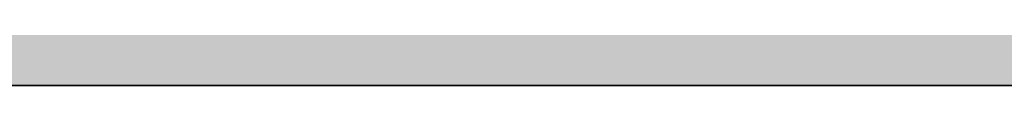
# Model space of a CAD drawing. Units: inches. Extents: x 2083 to 3317, y 1141 to 2115.
# Tile 133 of 256: x 3123.979 to 3126.132, y 1263.261 to 1263.355. Entities that reach past the tile are written whole.
import ezdxf

# ---------------------------------------------------------------- set-up
doc = ezdxf.new("R2010")
doc.units = ezdxf.units.IN
doc.layers.add('A-ANNO-DIMS', color=2, linetype='Continuous', lineweight=18)
doc.layers.add('A-WALL', color=7, linetype='Continuous', lineweight=35)
doc.layers.add('A-WALL-PATT', color=251, linetype='Continuous', lineweight=13, true_color=0x636466)
doc.styles.get("Standard").update_dxf_attribs({"font": 'arial.ttf'})
doc.dimstyles.new('ISO-25', dxfattribs={"dimtxt": 12, "dimasz": 12, "dimexe": 1.25, "dimexo": 0.625, "dimtad": 1, "dimlunit": 3, "dimtxsty": 'Standard', "dimcen": 2.5, "dimadec": 0, "dimazin": 0, "dimtfac": 1, "dimtmove": 0, "dimatfit": 3, "dimfxl": 1, "dimarcsym": 0})

# ---------------------------------------------------------------- blocks, each defined once
blk = doc.blocks.new('*D10')
at = {"layer": 'A-ANNO-DIMS', "color": 0, "lineweight": -2, "transparency": 16777216}
for p, q in [((2862.9598, 1262.6364), (2862.9598, 1201.3844)), ((3126.9598, 1262.6364), (3126.9598, 1201.3844)), ((2874.9598, 1202.6344), (3114.9598, 1202.6344))]:
    blk.add_line(p, q, dxfattribs=at)
at = {"layer": 'A-ANNO-DIMS', "color": 0, "transparency": 16777216}
for points in [[(2874.9598, 1204.6344), (2874.9598, 1200.6344), (2862.9598, 1202.6344)], [(3114.9598, 1204.6344), (3114.9598, 1200.6344), (3126.9598, 1202.6344)]]:
    blk.add_solid(points, dxfattribs=at)
at = {"layer": 'Defpoints', "color": 0, "transparency": 16777216}
for p in [(2862.9598, 1263.2614), (3126.9598, 1263.2614), (3126.9598, 1202.6344)]:
    blk.add_point(p, dxfattribs=at)
at = {"layer": 'A-ANNO-DIMS', "color": 0, "transparency": 16777216, "insert": (2994.9598, 1209.284), "char_height": 12, "attachment_point": 5}
blk.add_mtext("22'", dxfattribs=at)
blk = doc.blocks.new('*D26')
at = {"layer": 'A-ANNO-DIMS', "color": 0, "lineweight": -2, "transparency": 16777216}
for p, q in [((3088.9858, 1274.9151), (3088.9858, 1270.952)), ((3111.24, 1274.9151), (3111.24, 1270.952)), ((3076.9858, 1272.202), (2840.2624, 1272.202)), ((3111.24, 1272.202), (3088.9858, 1272.202)), ((3123.24, 1272.202), (3135.24, 1272.202))]:
    blk.add_line(p, q, dxfattribs=at)
at = {"layer": 'A-ANNO-DIMS', "color": 0, "transparency": 16777216}
for points in [[(3076.9858, 1274.202), (3076.9858, 1270.202), (3088.9858, 1272.202)], [(3123.24, 1274.202), (3123.24, 1270.202), (3111.24, 1272.202)]]:
    blk.add_solid(points, dxfattribs=at)
at = {"layer": 'Defpoints', "color": 0, "transparency": 16777216}
for p in [(3088.9858, 1275.5401), (3111.24, 1275.5401), (3088.9858, 1272.202)]:
    blk.add_point(p, dxfattribs=at)
at = {"layer": 'A-ANNO-DIMS', "color": 0, "transparency": 16777216, "insert": (2952.6241, 1279.0316), "char_height": 12, "attachment_point": 5}
blk.add_mtext('NIGHTSTAND 1\'-10 1/2" TYP.', dxfattribs=at)
blk = doc.blocks.new('*D27')
at = {"layer": 'A-ANNO-DIMS', "color": 0, "lineweight": -2, "transparency": 16777216}
for p, q in [((3114.5782, 1309.7943), (3114.5782, 1321.7943)), ((3111.865, 1297.7943), (3115.8282, 1297.7943)), ((3114.5782, 1297.7943), (3114.5782, 1275.5401)), ((3111.865, 1275.5401), (3115.8282, 1275.5401)), ((3114.5782, 1263.5401), (3114.5782, 1140.9886))]:
    blk.add_line(p, q, dxfattribs=at)
at = {"layer": 'A-ANNO-DIMS', "color": 0, "transparency": 16777216}
for points in [[(3112.5782, 1309.7943), (3116.5782, 1309.7943), (3114.5782, 1297.7943)], [(3112.5782, 1263.5401), (3116.5782, 1263.5401), (3114.5782, 1275.5401)]]:
    blk.add_solid(points, dxfattribs=at)
at = {"layer": 'Defpoints', "color": 0, "transparency": 16777216}
for p in [(3111.24, 1297.7943), (3111.24, 1275.5401), (3114.5782, 1275.5401)]:
    blk.add_point(p, dxfattribs=at)
at = {"layer": 'A-ANNO-DIMS', "color": 0, "transparency": 16777216, "insert": (3107.7485, 1196.2643), "char_height": 12, "attachment_point": 5, "rotation": 90}
blk.add_mtext('1\'-10 1/2" TYP.', dxfattribs=at)

msp = doc.modelspace()

# ---------------------------------------------------------------- hatches: boundary and pattern name
at = {"layer": 'A-WALL-PATT'}
h = msp.add_hatch(color=256, dxfattribs=at)
h.dxf.hatch_style = 1
h.paths.add_polyline_path([(3126.9598, 2020.7614), (2748.9598, 2020.7614), (2604.9598, 2020.7614), (2226.9598, 2020.7614), (2226.9598, 1702.7614), (2466.9598, 1702.7614), (2466.9598, 1582.7614), (2418.9598, 1582.7614), (2418.9598, 1477.7614), (2226.9598, 1477.7614), (2226.9598, 1263.2614), (2544.9598, 1263.2614), (2544.9598, 1411.7614), (2604.9598, 1411.7614), (2685.9598, 1411.7614), (2685.9598, 1420.7614), (2604.9598, 1420.7614), (2604.9598, 1573.7614), (2604.9598, 1702.7614), (2604.9598, 2011.7614), (2748.9598, 2011.7614), (2748.9598, 1702.7614), (2862.9598, 1702.7614), (2862.9598, 1621.7614), (2871.9598, 1621.7614), (2871.9598, 1702.7614), (2883.9598, 1702.7614), (2883.9598, 1706.9395, -0.026459), (2883.9598, 1711.7614), (2757.9598, 1711.7614), (2757.9598, 1807.7614), (2787.9598, 1807.7614), (2787.9598, 1812.2614), (2757.9598, 1812.2614), (2757.9598, 2011.7614), (2877.9598, 2011.7614), (2877.9598, 1812.2614), (2847.9598, 1812.2614), (2847.9598, 1807.7614), (2889.8357, 1807.7614), (2889.8357, 1812.2614), (2882.4598, 1812.2614), (2882.4598, 2011.7614), (3117.9598, 2011.7614), (3117.9598, 1812.2614), (2937.8357, 1812.2614), (2937.8357, 1807.7614), (2995.7098, 1807.7614), (2995.7098, 1796.1177), (3000.2098, 1796.1177), (3000.2098, 1807.7614), (3117.9598, 1807.7614), (3117.9598, 1711.7614), (3000.2098, 1711.7614), (3000.2098, 1760.1177), (2998.5727, 1760.1177, -0.020711), (2995.7098, 1760.1177), (2995.7098, 1711.7614), (2931.9598, 1711.7614), (2931.9598, 1702.7614), (3126.9598, 1702.7614)])
h.paths.add_polyline_path([(2471.4598, 2011.7614), (2471.4598, 1810.0114), (2462.7169, 1810.0114), (2462.7169, 1805.5114), (2505.9598, 1805.5114), (2505.9598, 1810.0114), (2475.9598, 1810.0114), (2475.9598, 2011.7614), (2595.9598, 2011.7614), (2595.9598, 1810.0114), (2565.9598, 1810.0114), (2565.9598, 1805.5114), (2595.9598, 1805.5114), (2595.9598, 1711.7614), (2235.9598, 1711.7614), (2235.9598, 1805.5114), (2353.7098, 1805.5114), (2353.7098, 1796.0542), (2358.2098, 1796.0542), (2358.2098, 1805.5114), (2414.7169, 1805.5114), (2414.7169, 1810.0114), (2235.9598, 1810.0114), (2235.9598, 2011.7614)], flags=16)
h.paths.add_polyline_path([(2270.2047, 1994.61), (2270.2047, 1970.61), (2246.2047, 1970.61), (2246.2047, 1994.61)], flags=0)
edge = h.paths.add_edge_path(flags=0)
edge.add_ellipse((2332.0274, 1899.7982), major_axis=(-3.043, 3.043), ratio=0.168252, start_angle=-161.3322, end_angle=-156.3071, ccw=False)
edge.add_ellipse((2333.082, 1898.7435), major_axis=(-1.0546, 1.0546), ratio=0.453532, start_angle=-123.371, end_angle=-94.1591)
edge = h.paths.add_edge_path(flags=0)
edge.add_ellipse((2332.0274, 1968.8763), major_axis=(3.043, 3.043), ratio=0.168252, start_angle=18.6678, end_angle=23.6929)
edge.add_spline(control_points=[(2332.9256, 1970.6911), (2332.2268, 1970.3361), (2330.8937, 1969.6589), (2328.4131, 1970.9321), (2327.2039, 1967.7487), (2324.7096, 1969.9556), (2322.5328, 1967.0124), (2320.0128, 1971.2958), (2317.6803, 1968.1578), (2316.0405, 1967.102), (2315.4269, 1966.8096)], knot_values=[0, 0, 0, 0, 2.267059, 4.324559, 6.685584, 8.878641, 11.121502, 14.300359, 17.755284, 19.732645, 19.732645, 19.732645, 19.732645], degree=3, periodic=0)
edge.add_ellipse((2332.0274, 1968.8763), major_axis=(3.043, 3.043), ratio=0.168252, start_angle=18.6678, end_angle=23.6929, ccw=False)
edge.add_ellipse((2333.082, 1969.9309), major_axis=(1.0546, 1.0546), ratio=0.453532, start_angle=56.629, end_angle=85.8409, ccw=False)
edge = h.paths.add_edge_path(flags=0)
edge.add_spline(control_points=[(2296.4283, 1967.9879), (2293.6278, 1965.3363), (2287.7036, 1959.7271), (2299.7439, 1949.9957), (2294.5326, 1935.6685), (2290.5732, 1920.6035), (2293.3941, 1909.9737), (2296.1854, 1904.9665)], knot_values=[0.099185, 0.099185, 0.099185, 0.099185, 0.345301, 0.619822, 0.982653, 1.386093, 1.810555, 1.810555, 1.810555, 1.810555], degree=3, periodic=0)
edge.add_spline(control_points=[(2296.1854, 1904.9665), (2297.3836, 1902.6193), (2298.001, 1901.9493), (2298.553, 1901.4682)], knot_values=[0.006246, 0.006246, 0.006246, 0.006246, 0.055476, 0.055476, 0.055476, 0.055476], degree=3, periodic=0)
edge.add_spline(control_points=[(2298.553, 1901.4682), (2297.2586, 1900.9232), (2295.2253, 1900.2321), (2293.0602, 1900.6142), (2292.1014, 1900.7884), (2292.0896, 1900.7906)], knot_values=[0.312835, 0.312835, 0.312835, 0.312835, 0.40178, 0.474987, 0.475903, 0.475903, 0.475903, 0.475903], degree=3, periodic=0)
edge.add_arc((2292.7936, 1904.6641), 3.937, 215.4209, 259.6982, ccw=False)
edge.add_spline(control_points=[(2289.5853, 1902.3823), (2289.4767, 1902.5351), (2289.3685, 1902.688), (2289.2609, 1902.8412)], knot_values=[0.102872, 0.102872, 0.102872, 0.102872, 0.116896, 0.116896, 0.116896, 0.116896], degree=3, periodic=0)
edge.add_spline(control_points=[(2289.2609, 1902.8412), (2288.6866, 1902.5502), (2287.64, 1902.0199), (2285.8813, 1901.874), (2283.853, 1901.5044), (2281.72, 1899.7105), (2278.467, 1899.4929), (2276.1571, 1901.8832), (2272.259, 1899.8041), (2267.7776, 1901.8432), (2262.2439, 1900.184), (2257.4149, 1901.7821), (2254.3184, 1900.7261), (2253.1783, 1900.3373)], knot_values=[0, 0, 0, 0, 1.907977, 3.477176, 5.261074, 7.972851, 11.680248, 13.717921, 16.939592, 22.789562, 27.502503, 33.595215, 37.145618, 37.145618, 37.145618, 37.145618], degree=3, periodic=0)
edge.add_line((2253.1783, 1900.3373), (2250.2442, 1902.8412))
edge.add_line((2250.2442, 1902.8412), (2250.2442, 1965.8333))
edge.add_line((2250.2442, 1965.8333), (2253.1783, 1968.3371))
edge.add_spline(control_points=[(2253.1783, 1968.3371), (2254.3184, 1967.9483), (2257.4149, 1966.8924), (2262.2439, 1968.4904), (2267.7776, 1966.8313), (2271.5267, 1968.5372), (2273.8759, 1967.8283), (2274.2067, 1967.7276)], knot_values=[0, 0, 0, 0, 0.09018, 0.244935, 0.364644, 0.513233, 0.537855, 0.537855, 0.537855, 0.537855], degree=3, periodic=0)
edge.add_arc((2274.3529, 1963.7933), 3.937, 72.0511, 92.1279, ccw=False)
edge.add_arc((2281.2969, 1985.23), 18.5963, 252.05113, 288.56572)
edge.add_arc((2292.3167, 1956.0289), 12.6461, 71.02679, 113.77822, ccw=False)
edge = h.paths.add_edge_path(flags=0)
edge.add_spline(control_points=[(2274.8994, 1951.8562), (2275.0662, 1951.6166), (2275.2327, 1951.3766), (2275.398, 1951.1359)], knot_values=[1.409916, 1.409916, 1.409916, 1.409916, 1.43159, 1.43159, 1.43159, 1.43159], degree=3, periodic=0)
edge.add_spline(control_points=[(2275.398, 1951.1359), (2275.7921, 1950.5619), (2276.1792, 1949.9838), (2276.5455, 1949.3971)], knot_values=[1.358238, 1.358238, 1.358238, 1.358238, 1.409916, 1.409916, 1.409916, 1.409916], degree=3, periodic=0)
edge.add_line((2276.5455, 1949.3971), (2277.4373, 1947.8622))
edge.add_spline(control_points=[(2277.4373, 1947.8622), (2276.3038, 1945.6731), (2274.6397, 1942.4269), (2274.6316, 1938.0939), (2272.7991, 1930.8515), (2274.3564, 1943.897), (2275.9477, 1947.9234), (2276.5455, 1949.3971)], knot_values=[0.005632, 0.005632, 0.005632, 0.005632, 0.186014, 0.266002, 0.357087, 0.59639, 0.739732, 0.739732, 0.739732, 0.739732], degree=3, periodic=0)
edge.add_spline(control_points=[(2276.5455, 1949.3971), (2276.1792, 1949.9838), (2275.7921, 1950.5619), (2275.398, 1951.1359)], knot_values=[1.358238, 1.358238, 1.358238, 1.358238, 1.409916, 1.409916, 1.409916, 1.409916], degree=3, periodic=0)
edge.add_spline(control_points=[(2275.398, 1951.1359), (2274.9425, 1950.0805), (2274.2078, 1948.0253), (2273.9346, 1944.8515), (2272.4685, 1937.6275), (2273.4662, 1945.6965), (2274.7006, 1951.0595), (2274.8994, 1951.8562)], knot_values=[0.104364, 0.104364, 0.104364, 0.104364, 0.189636, 0.269624, 0.36071, 0.600013, 0.644622, 0.644622, 0.644622, 0.644622], degree=3, periodic=0)
h.paths.add_polyline_path([(2269.1675, 1963.1276, -0.357527), (2268.1706, 1960.9764, -0.092561), (2268.1706, 1939.4363, -0.357527), (2269.1675, 1937.2851, -0.357527), (2267.0163, 1938.282, -0.164785), (2254.6856, 1938.282, -0.357527), (2252.5344, 1937.2851, -0.357527), (2253.5313, 1939.4363, -0.092561), (2253.5313, 1960.9764, -0.357527), (2252.5344, 1963.1276, -0.357527), (2254.6856, 1962.1307, -0.164785), (2267.0163, 1962.1307, -0.357527)], flags=0)
h.paths.add_polyline_path([(2248.8741, 1967.8018), (2248.8741, 1957.0277), (2249.4578, 1957.0277), (2249.4578, 1911.6468), (2248.8741, 1911.6468), (2248.8741, 1900.8727), (2246.5119, 1900.8727, 0.197327), (2244.1497, 1902.4569), (2244.1497, 1966.2176, 0.197327), (2246.5119, 1967.8018)], flags=0)
h.paths.add_polyline_path([(2269.1675, 1931.3893, -0.357527), (2268.1706, 1929.2381, -0.092561), (2268.1706, 1907.6981, -0.357527), (2269.1675, 1905.5469, -0.357527), (2267.0163, 1906.5438, -0.164785), (2254.6856, 1906.5438, -0.357527), (2252.5344, 1905.5469, -0.357527), (2253.5313, 1907.6981, -0.092561), (2253.5313, 1929.2381, -0.357527), (2252.5344, 1931.3893, -0.357527), (2254.6856, 1930.3925, -0.164785), (2267.0163, 1930.3925, -0.357527)], flags=0)
edge = h.paths.add_edge_path(flags=0)
edge.add_spline(control_points=[(2276.1969, 1906.7237), (2276.1681, 1909.0289), (2276.114, 1913.3719), (2270.5984, 1924.925), (2273.9052, 1919.0128), (2275.9217, 1916.2621), (2275.4746, 1912.4021), (2277.2579, 1910.3806), (2276.696, 1908.225), (2276.6462, 1906.813), (2276.6178, 1906.0084)], knot_values=[0, 0, 0, 0, 8.61026, 16.221274, 18.843057, 23.804898, 27.440828, 29.356102, 31.203478, 33.650687, 33.650687, 33.650687, 33.650687], degree=3, periodic=0)
edge.add_spline(control_points=[(2276.6178, 1906.0084), (2276.6233, 1905.6241), (2276.4977, 1904.6287), (2275.4418, 1903.8547), (2274.9373, 1903.0804), (2274.8591, 1902.8412)], knot_values=[0.156488, 0.156488, 0.156488, 0.156488, 0.184398, 0.231376, 0.250598, 0.250598, 0.250598, 0.250598], degree=3, periodic=0)
edge.add_line((2274.8591, 1902.8412), (2276.506, 1902.8412))
edge.add_spline(control_points=[(2276.506, 1902.8412), (2276.7883, 1903.0849), (2277.6651, 1904.1252), (2278.2495, 1904.3407), (2277.6539, 1908.5274), (2278.1557, 1906.2278), (2278.1005, 1905.2859), (2278.8467, 1904.069), (2277.8568, 1903.4149), (2277.8742, 1902.991), (2277.9036, 1902.8412)], knot_values=[0.059574, 0.059574, 0.059574, 0.059574, 0.080753, 0.103741, 0.16972, 0.176036, 0.207137, 0.240474, 0.262341, 0.27366, 0.27366, 0.27366, 0.27366], degree=3, periodic=0)
edge.add_line((2277.9036, 1902.8412), (2280.0298, 1902.8412))
edge.add_spline(control_points=[(2280.0298, 1902.8412), (2279.8882, 1903.0884), (2279.4993, 1903.9816), (2280.1523, 1905.9393), (2278.1036, 1909.6578), (2279.7624, 1907.1853), (2280.3279, 1904.8749), (2280.4851, 1903.4896), (2281.4633, 1903.2494), (2281.7583, 1902.9365), (2281.834, 1902.8412)], knot_values=[0.013856, 0.013856, 0.013856, 0.013856, 0.034874, 0.088867, 0.107879, 0.126738, 0.158714, 0.193757, 0.217487, 0.226722, 0.226722, 0.226722, 0.226722], degree=3, periodic=0)
edge.add_spline(control_points=[(2281.834, 1902.8412), (2281.7875, 1902.8267), (2281.647, 1902.783), (2281.3955, 1902.8595), (2281.0881, 1902.9852), (2280.7207, 1903.0609), (2280.3335, 1903.0257), (2280.1248, 1902.8989), (2280.0298, 1902.8412)], knot_values=[0, 0, 0, 0, 0.14413, 0.435517, 0.749276, 1.153046, 1.548371, 1.878348, 1.878348, 1.878348, 1.878348], degree=3, periodic=0)
edge.add_line((2280.0298, 1902.8412), (2277.9036, 1902.8412))
edge.add_spline(control_points=[(2277.9036, 1902.8412), (2277.8929, 1902.7959), (2277.8654, 1902.6796), (2277.6075, 1902.6875), (2277.2741, 1902.8007), (2276.8379, 1902.6198), (2276.5838, 1902.7893), (2276.506, 1902.8412)], knot_values=[0, 0, 0, 0, 0.127189, 0.326199, 0.628009, 1.24357, 1.515331, 1.515331, 1.515331, 1.515331], degree=3, periodic=0)
edge.add_line((2276.506, 1902.8412), (2274.8591, 1902.8412))
edge.add_spline(control_points=[(2274.8591, 1902.8412), (2274.8144, 1902.8986), (2274.7251, 1903.0134), (2274.4935, 1903.119), (2274.2443, 1902.9605), (2273.9371, 1903.1849), (2273.614, 1902.9831), (2273.4083, 1902.883), (2273.3223, 1902.8412)], knot_values=[0, 0, 0, 0, 0.21843, 0.436957, 0.687977, 0.990379, 1.398396, 1.69185, 1.69185, 1.69185, 1.69185], degree=3, periodic=0)
edge.add_spline(control_points=[(2273.3223, 1902.8412), (2273.6167, 1903.4457), (2274.274, 1904.5383), (2276.0272, 1904.5737), (2276.207, 1906.5836), (2276.1969, 1906.7237)], knot_values=[0.012227, 0.012227, 0.012227, 0.012227, 0.059472, 0.106218, 0.134458, 0.134458, 0.134458, 0.134458], degree=3, periodic=0)
h.paths.add_polyline_path([(2270.7761, 1897.7898), (2270.7761, 1873.7898), (2246.7761, 1873.7898), (2246.7761, 1897.7898)], flags=0)
h.paths.add_polyline_path([(2353.7098, 1760.0051), (2353.7098, 1760.0542), (2358.2098, 1760.0542, -0.033729)], flags=0)
h.paths.add_polyline_path([(2321.8191, 1737.5292), (2341.9953, 1737.5292, -0.414214), (2343.2033, 1736.3212), (2343.2033, 1721.0206, -0.414214), (2341.9953, 1719.8127), (2321.8191, 1719.8127, -0.414214), (2320.6112, 1721.0206), (2320.6112, 1736.3212, -0.414214)], flags=0)
h.paths.add_polyline_path([(2324.235, 1736.3212), (2339.5794, 1736.3212, -0.414214), (2341.9953, 1733.9053), (2341.9953, 1725.4497, -0.414214), (2339.5794, 1723.0338), (2333.6806, 1723.0338), (2333.8453, 1722.0455, -0.870646), (2335.4254, 1721.8259, -0.767327), (2333.9227, 1721.4232), (2331.291, 1721.4232, -0.767327), (2329.7883, 1721.8259, -0.870646), (2331.3684, 1722.0455), (2331.5331, 1723.0338), (2324.235, 1723.0338, -0.414214), (2321.8191, 1725.4497), (2321.8191, 1733.9053, -0.414214)], flags=0)
h.paths.add_polyline_path([(2570.4838, 1928.6154), (2589.6838, 1928.6154), (2590.1688, 1928.6154), (2590.1688, 1904.9934), (2570.4838, 1904.9934)], flags=0)
h.paths.add_polyline_path([(2574.4473, 1927.2638, -1), (2572.8288, 1927.2638, -1)], flags=0)
h.paths.add_polyline_path([(2573.0899, 1926.9409), (2573.925, 1927.776), (2574.1477, 1927.5533), (2573.3126, 1926.7182)], flags=0)
h.paths.add_polyline_path([(2578.7791, 1919.7296, -1), (2571.5917, 1919.7296, -1)], flags=0)
h.paths.add_polyline_path([(2578.3854, 1919.7296, -1), (2571.9854, 1919.7296, -1)], flags=0)
h.paths.add_polyline_path([(2331.5958, 1729.4762, -1), (2333.618, 1729.4762, -1)], flags=0)
h.paths.add_polyline_path([(2578.0342, 1927.2638, -1), (2576.4157, 1927.2638, -1)], flags=0)
h.paths.add_polyline_path([(2576.6889, 1927.5311), (2576.9116, 1927.7538), (2577.7467, 1926.9186), (2577.524, 1926.6959)], flags=0)
h.paths.add_polyline_path([(2578.1391, 1909.8595, -1), (2572.2317, 1909.8595, -1)], flags=0)
h.paths.add_polyline_path([(2577.7454, 1909.8595, -1), (2572.6254, 1909.8595, -1)], flags=0)
h.paths.add_polyline_path([(2583.7977, 1927.2638, -1), (2582.1792, 1927.2638, -1)], flags=0)
h.paths.add_polyline_path([(2582.7186, 1927.7538), (2583.5538, 1926.9186), (2583.3311, 1926.6959), (2582.4959, 1927.5311)], flags=0)
h.paths.add_polyline_path([(2582.4959, 1927.5311), (2582.7186, 1927.7538), (2583.5538, 1926.9186), (2583.3311, 1926.6959)], flags=0)
h.paths.add_polyline_path([(2587.7391, 1920.5296, -1), (2581.8317, 1920.5296, -1)], flags=0)
h.paths.add_polyline_path([(2587.3454, 1920.5296, -1), (2582.2254, 1920.5296, -1)], flags=0)
h.paths.add_polyline_path([(2587.3846, 1927.2638, -1), (2585.7661, 1927.2638, -1)], flags=0)
h.paths.add_polyline_path([(2586.082, 1926.9802), (2586.9172, 1927.8154), (2587.1399, 1927.5927), (2586.3047, 1926.7575)], flags=0)
h.paths.add_polyline_path([(2588.3791, 1910.6595, -1), (2581.1917, 1910.6595, -1)], flags=0)
h.paths.add_polyline_path([(2587.9854, 1910.6595, -1), (2581.5854, 1910.6595, -1)], flags=0)
h.paths.add_polyline_path([(2417.1677, 1729.4779), (2437.3439, 1729.4779, -0.414214), (2438.5519, 1728.2699), (2438.5519, 1712.9693, -0.414214), (2437.3439, 1711.7614), (2417.1677, 1711.7614, -0.414214), (2415.9598, 1712.9693), (2415.9598, 1728.2699, -0.414214)], flags=0)
h.paths.add_polyline_path([(2419.5836, 1728.2699), (2434.928, 1728.2699, -0.414214), (2437.3439, 1725.8541), (2437.3439, 1717.3984, -0.414214), (2434.928, 1714.9825), (2429.0292, 1714.9825), (2429.1939, 1713.9942, -0.870646), (2430.774, 1713.7746, -0.767327), (2429.2713, 1713.372), (2426.6396, 1713.372, -0.767327), (2425.1369, 1713.7746, -0.870646), (2426.717, 1713.9942), (2426.8817, 1714.9825), (2419.5836, 1714.9825, -0.414214), (2417.1677, 1717.3984), (2417.1677, 1725.8541, -0.414214)], flags=0)
h.paths.add_polyline_path([(2419.5836, 1728.2699), (2434.928, 1728.2699, -0.414214), (2437.3439, 1725.8541), (2437.3439, 1717.3984, -0.414214), (2434.928, 1714.9825), (2429.0292, 1714.9825), (2428.3581, 1719.009), (2427.5528, 1719.009), (2426.8817, 1714.9825), (2419.5836, 1714.9825, -0.414214), (2417.1677, 1717.3984), (2417.1677, 1725.8541, -0.414214)], flags=0)
h.paths.add_polyline_path([(2426.9444, 1721.4249, -1), (2428.9666, 1721.4249, -1)], flags=0)
h.paths.add_polyline_path([(2475.9598, 1702.7614), (2595.9598, 1702.7614), (2595.9598, 1582.7614), (2475.9598, 1582.7614)], flags=16)
h.paths.add_polyline_path([(2427.9598, 1573.7614), (2595.9598, 1573.7614), (2595.9598, 1468.7614), (2595.9598, 1420.7614), (2384.4598, 1420.7614), (2384.4598, 1468.7614), (2427.9598, 1468.7614)], flags=16)
h.paths.add_polyline_path([(2379.9598, 1468.7614), (2379.9598, 1420.7614), (2235.9598, 1420.7614), (2235.9598, 1468.7614)], flags=16)
h.paths.add_polyline_path([(2317.816, 1466.6958), (2337.9922, 1466.6958, -0.414214), (2339.2002, 1465.4878), (2339.2002, 1450.1872, -0.414214), (2337.9922, 1448.9792), (2317.816, 1448.9792, -0.414214), (2316.6081, 1450.1872), (2316.6081, 1465.4878, -0.414214)], flags=0)
h.paths.add_polyline_path([(2320.2319, 1465.4878), (2335.5763, 1465.4878, -0.414214), (2337.9922, 1463.0719), (2337.9922, 1454.6163, -0.414214), (2335.5763, 1452.2004), (2329.6775, 1452.2004), (2329.8422, 1451.212, -0.870646), (2331.4223, 1450.9925, -0.767327), (2329.9196, 1450.5898), (2327.2879, 1450.5898, -0.767327), (2325.7852, 1450.9925, -0.870646), (2327.3653, 1451.212), (2327.53, 1452.2004), (2320.2319, 1452.2004, -0.414214), (2317.816, 1454.6163), (2317.816, 1463.0719, -0.414214)], flags=0)
h.paths.add_polyline_path([(2320.2319, 1465.4878), (2335.5763, 1465.4878, -0.414214), (2337.9922, 1463.0719), (2337.9922, 1454.6163, -0.414214), (2335.5763, 1452.2004), (2329.6775, 1452.2004), (2329.0064, 1456.2269), (2328.2011, 1456.2269), (2327.53, 1452.2004), (2320.2319, 1452.2004, -0.414214), (2317.816, 1454.6163), (2317.816, 1463.0719, -0.414214)], flags=0)
h.paths.add_polyline_path([(2327.5926, 1458.6428, -1), (2329.6148, 1458.6428, -1)], flags=0)
h.paths.add_polyline_path([(2244.4117, 1433.3405), (2241.9209, 1433.3405, -0.414214), (2240.0179, 1435.2435), (2240.0179, 1440.9528, -0.414211), (2241.9209, 1442.8559), (2244.4117, 1442.8559, -1.976472)], flags=0)
h.paths.add_polyline_path([(2245.3569, 1434.3975, -0.414214), (2245.3569, 1441.7988, -2.144098)], flags=0)
h.paths.add_polyline_path([(2535.9598, 1416.2614), (2535.9598, 1272.2614), (2235.9598, 1272.2614), (2235.9598, 1416.2614)], flags=16)
h.paths.add_polyline_path([(2260.1196, 1384.2928), (2260.1196, 1362.0386), (2237.8654, 1362.0386), (2237.8654, 1384.2928)], flags=0)
edge = h.paths.add_edge_path(flags=0)
edge.add_line((2318.2518, 1362.0933), (2318.1458, 1362.001))
edge.add_ellipse((2317.4451, 1360.431), major_axis=(2.8216, 2.8216), ratio=0.168252, start_angle=18.6678, end_angle=20.9481, ccw=False)
edge.add_ellipse((2318.423, 1361.409), major_axis=(0.9779, 0.9779), ratio=0.453532, start_angle=56.629, end_angle=70.2262, ccw=False)
edge = h.paths.add_edge_path(flags=0)
edge.add_line((2319.1074, 1295.5711), (2319.015, 1295.6771))
edge.add_ellipse((2317.4451, 1296.3778), major_axis=(-2.8216, 2.8216), ratio=0.168252, start_angle=-161.3322, end_angle=-159.0519, ccw=False)
edge.add_ellipse((2318.423, 1295.3999), major_axis=(-0.9779, 0.9779), ratio=0.453532, start_angle=-123.371, end_angle=-109.7738)
edge = h.paths.add_edge_path(flags=0)
edge.add_spline(control_points=[(2284.2103, 1301.1702), (2284.5807, 1300.4447), (2284.8912, 1299.892), (2285.1596, 1299.461)], knot_values=[0.039066, 0.039066, 0.039066, 0.039066, 0.055476, 0.055476, 0.055476, 0.055476], degree=3, periodic=0)
edge.add_line((2285.1596, 1299.461), (2284.2103, 1301.1702))
edge = h.paths.add_edge_path(flags=0)
edge.add_line((2280.4125, 1297.298), (2283.37, 1297.0361))
edge.add_line((2283.37, 1297.0361), (2286.4057, 1297.9263))
edge.add_spline(control_points=[(2286.4057, 1297.9263), (2285.3055, 1297.4631), (2284.3448, 1297.1292), (2283.37, 1297.0361)], knot_values=[0.394369, 0.394369, 0.394369, 0.394369, 0.475903, 0.475903, 0.475903, 0.475903], degree=3, periodic=0)
edge.add_spline(control_points=[(2283.37, 1297.0361), (2283.2814, 1297.0277), (2282.3163, 1296.9573), (2281.3125, 1297.1345), (2280.4234, 1297.296), (2280.4125, 1297.298)], knot_values=[0.312835, 0.312835, 0.312835, 0.312835, 0.320246, 0.393453, 0.394369, 0.394369, 0.394369, 0.394369], degree=3, periodic=0)
edge = h.paths.add_edge_path(flags=0)
edge.add_line((2284.4356, 1359.6073), (2280.4463, 1355.328))
edge.add_line((2280.4463, 1355.328), (2279.58, 1351.0178))
edge.add_line((2279.58, 1351.0178), (2282.413, 1346.5804))
edge.add_spline(control_points=[(2282.413, 1346.5804), (2283.1533, 1345.5892), (2284.2529, 1344.0289), (2284.801, 1342.3872), (2284.9352, 1341.8055)], knot_values=[1.240098, 1.240098, 1.240098, 1.240098, 1.332892, 1.382712, 1.382712, 1.382712, 1.382712], degree=3, periodic=0)
edge.add_spline(control_points=[(2284.9352, 1341.8055), (2285.3191, 1340.1406), (2285.233, 1338.4092), (2284.9099, 1336.6541)], knot_values=[1.097484, 1.097484, 1.097484, 1.097484, 1.240098, 1.240098, 1.240098, 1.240098], degree=3, periodic=0)
edge.add_spline(control_points=[(2284.9099, 1336.6541), (2284.5868, 1334.899), (2284.0267, 1333.1203), (2283.4626, 1331.3606)], knot_values=[0.95487, 0.95487, 0.95487, 0.95487, 1.097484, 1.097484, 1.097484, 1.097484], degree=3, periodic=0)
edge.add_line((2283.4626, 1331.3606), (2281.8904, 1326.1534))
edge.add_line((2281.8904, 1326.1534), (2280.7563, 1321.0561))
edge.add_line((2280.7563, 1321.0561), (2280.2992, 1316.002))
edge.add_line((2280.2992, 1316.002), (2280.7159, 1310.9501))
edge.add_line((2280.7159, 1310.9501), (2282.0281, 1305.9721))
edge.add_line((2282.0281, 1305.9721), (2284.2103, 1301.1702))
edge.add_spline(control_points=[(2284.2103, 1301.1702), (2283.3407, 1302.7302), (2282.6119, 1304.3365), (2282.0281, 1305.9721)], knot_values=[0.099185, 0.099185, 0.099185, 0.099185, 0.241799, 0.241799, 0.241799, 0.241799], degree=3, periodic=0)
edge.add_spline(control_points=[(2282.0281, 1305.9721), (2281.4443, 1307.6078), (2281.0055, 1309.2728), (2280.7159, 1310.9501)], knot_values=[0.241799, 0.241799, 0.241799, 0.241799, 0.384413, 0.384413, 0.384413, 0.384413], degree=3, periodic=0)
edge.add_spline(control_points=[(2280.7159, 1310.9501), (2280.4332, 1312.5876), (2280.2894, 1314.277), (2280.2989, 1315.962), (2280.2992, 1316.002)], knot_values=[0.384413, 0.384413, 0.384413, 0.384413, 0.523647, 0.527028, 0.527028, 0.527028, 0.527028], degree=3, periodic=0)
edge.add_spline(control_points=[(2280.2992, 1316.002), (2280.3123, 1317.687), (2280.4779, 1319.3679), (2280.7563, 1321.0561)], knot_values=[0.527028, 0.527028, 0.527028, 0.527028, 0.669642, 0.669642, 0.669642, 0.669642], degree=3, periodic=0)
edge.add_spline(control_points=[(2280.7563, 1321.0561), (2281.0346, 1322.7443), (2281.4259, 1324.4396), (2281.8904, 1326.1534)], knot_values=[0.669642, 0.669642, 0.669642, 0.669642, 0.812256, 0.812256, 0.812256, 0.812256], degree=3, periodic=0)
edge.add_spline(control_points=[(2281.8904, 1326.1534), (2282.2644, 1327.5333), (2282.7879, 1329.2618), (2283.3528, 1331.0178), (2283.4626, 1331.3606)], knot_values=[0.812256, 0.812256, 0.812256, 0.812256, 0.927087, 0.95487, 0.95487, 0.95487, 0.95487], degree=3, periodic=0)
edge.add_line((2283.4626, 1331.3606), (2284.9099, 1336.6541))
edge.add_line((2284.9099, 1336.6541), (2284.9352, 1341.8055))
edge.add_line((2284.9352, 1341.8055), (2282.413, 1346.5804))
edge.add_spline(control_points=[(2282.413, 1346.5804), (2281.2751, 1348.1038), (2280.0784, 1349.5703), (2279.58, 1351.0178)], knot_values=[1.382712, 1.382712, 1.382712, 1.382712, 1.525326, 1.525326, 1.525326, 1.525326], degree=3, periodic=0)
edge.add_spline(control_points=[(2279.58, 1351.0178), (2279.4433, 1351.4147), (2279.1363, 1352.8569), (2279.7352, 1354.2904), (2280.4463, 1355.328)], knot_values=[1.525326, 1.525326, 1.525326, 1.525326, 1.564439, 1.667941, 1.667941, 1.667941, 1.667941], degree=3, periodic=0)
edge.add_spline(control_points=[(2280.4463, 1355.328), (2281.4261, 1356.7578), (2282.9308, 1358.1826), (2284.4356, 1359.6073)], knot_values=[1.667941, 1.667941, 1.667941, 1.667941, 1.810555, 1.810555, 1.810555, 1.810555], degree=3, periodic=0)
edge.add_arc((2280.6231, 1348.5182), 11.7262, 71.02679, 113.77822)
edge.add_arc((2270.4049, 1375.5952), 17.2436, 252.05113, 288.56572, ccw=False)
edge.add_arc((2263.966, 1355.7178), 3.6506, 72.0511, 92.1279)
edge.add_arc((2263.966, 1355.7178), 3.6506, 92.1279, 177.9851)
edge.add_spline(control_points=[(2260.3176, 1355.8462), (2260.2604, 1354.2207), (2260.5513, 1350.1865), (2262.9993, 1346.7663), (2264.4727, 1344.649)], knot_values=[1.43159, 1.43159, 1.43159, 1.43159, 1.564144, 1.770695, 1.770695, 1.770695, 1.770695], degree=3, periodic=0)
edge.add_line((2264.4727, 1344.649), (2264.9356, 1343.9825))
edge.add_spline(control_points=[(2263.801, 1340.2481), (2263.8432, 1340.5141), (2264.0672, 1341.7565), (2264.5127, 1343.0025), (2264.935, 1343.9811)], knot_values=[0.53657, 0.53657, 0.53657, 0.53657, 0.559349, 0.644622, 0.644622, 0.644622, 0.644622], degree=3, periodic=0)
edge.add_spline(control_points=[(2264.935, 1343.9811), (2265.1178, 1343.715), (2265.2989, 1343.4479), (2265.4768, 1343.1794)], knot_values=[1.384077, 1.384077, 1.384077, 1.384077, 1.409916, 1.409916, 1.409916, 1.409916], degree=3, periodic=0)
edge.add_spline(control_points=[(2265.4768, 1343.1794), (2265.6546, 1342.9108), (2265.8293, 1342.6408), (2265.9991, 1342.3688)], knot_values=[1.358238, 1.358238, 1.358238, 1.358238, 1.384077, 1.384077, 1.384077, 1.384077], degree=3, periodic=0)
edge.add_line((2265.9991, 1342.3688), (2266.826, 1340.9455))
edge.add_spline(control_points=[(2266.826, 1340.9455), (2268.8944, 1337.0897), (2271.3982, 1325.843), (2270.5162, 1310.5686), (2275.9194, 1301.8606), (2277.7895, 1299.1994)], knot_values=[0.116896, 0.116896, 0.116896, 0.116896, 0.472987, 1.050969, 1.313793, 1.313793, 1.313793, 1.313793], degree=3, periodic=0)
edge.add_spline(control_points=[(2277.7895, 1299.1994), (2277.8394, 1299.1285), (2277.8894, 1299.0575), (2277.9396, 1298.9866)], knot_values=[0.109884, 0.109884, 0.109884, 0.109884, 0.116896, 0.116896, 0.116896, 0.116896], degree=3, periodic=0)
edge.add_line((2277.9396, 1298.9866), (2277.7888, 1299.1991))
edge.add_spline(control_points=[(2277.7888, 1299.1991), (2277.2566, 1298.9294), (2276.2864, 1298.4379), (2275.0394, 1298.3344), (2274.3833, 1298.2389), (2274.2153, 1298.2093)], knot_values=[33.12187, 33.12187, 33.12187, 33.12187, 35.029056, 36.598255, 37.144827, 37.144827, 37.144827, 37.144827], degree=3, periodic=0)
edge.add_line((2274.2153, 1298.2093), (2273.0731, 1297.893))
edge.add_spline(control_points=[(2273.0731, 1297.893), (2272.3229, 1297.5798), (2271.0392, 1296.5105), (2269.2484, 1296.2261), (2268.4231, 1296.3747)], knot_values=[26.532584, 26.532584, 26.532584, 26.532584, 29.198919, 31.839101, 31.839101, 31.839101, 31.839101], degree=3, periodic=0)
edge.add_line((2268.4231, 1296.3747), (2263.8785, 1297.4575))
edge.add_spline(control_points=[(2263.8785, 1297.4575), (2263.5561, 1297.3594), (2261.8603, 1296.8387), (2260.2388, 1297.2824), (2258.9335, 1297.5165)], knot_values=[15.919551, 15.919551, 15.919551, 15.919551, 16.939592, 21.226067, 21.226067, 21.226067, 21.226067], degree=3, periodic=0)
edge.add_line((2258.9335, 1297.5165), (2254.0552, 1297.329))
edge.add_spline(control_points=[(2254.0552, 1297.329), (2253.7555, 1297.2958), (2252.1137, 1297.1652), (2250.4619, 1297.5442), (2249.1297, 1297.6679)], knot_values=[5.306517, 5.306517, 5.306517, 5.306517, 6.276435, 10.613034, 10.613034, 10.613034, 10.613034], degree=3, periodic=0)
edge.add_line((2249.1297, 1297.6679), (2244.3316, 1296.8778))
edge.add_line((2244.3316, 1296.8778), (2241.611, 1299.1994))
edge.add_line((2241.611, 1299.1994), (2241.611, 1357.6094))
edge.add_line((2241.611, 1357.6094), (2244.3316, 1359.9311))
edge.add_line((2244.3316, 1359.9311), (2252.7288, 1359.5427))
edge.add_spline(control_points=[(2252.7288, 1359.5427), (2252.8709, 1359.5464), (2253.3057, 1359.5482), (2253.7398, 1359.5143), (2254.0317, 1359.4824)], knot_values=[0.233291, 0.233291, 0.233291, 0.233291, 0.244935, 0.268927, 0.268927, 0.268927, 0.268927], degree=3, periodic=0)
edge.add_line((2254.0317, 1359.4824), (2259.5872, 1359.4164))
edge.add_spline(control_points=[(2259.5872, 1359.4164), (2260.6771, 1359.6285), (2262.0732, 1359.897), (2263.5237, 1359.4593), (2263.8304, 1359.366)], knot_values=[0.422516, 0.422516, 0.422516, 0.422516, 0.513233, 0.537855, 0.537855, 0.537855, 0.537855], degree=3, periodic=0)
edge.add_arc((2263.966, 1355.7178), 3.6506, 72.0511, 92.1279, ccw=False)
edge.add_arc((2270.4049, 1375.5952), 17.2436, 252.05113, 288.56572)
edge.add_arc((2280.6231, 1348.5182), 11.7262, 71.02679, 113.77822, ccw=False)
h.paths.add_polyline_path([(2240.3405, 1359.4347), (2240.3405, 1349.4444), (2240.8818, 1349.4444), (2240.8818, 1307.3645), (2240.3405, 1307.3645), (2240.3405, 1297.3741), (2238.1502, 1297.3741, 0.197327), (2235.9598, 1298.8431), (2235.9598, 1357.9657, 0.197327), (2238.1502, 1359.4347)], flags=0)
h.paths.add_polyline_path([(2259.1578, 1355.1005, -0.357527), (2258.2334, 1353.1058, -0.092561), (2258.2334, 1333.1326, -0.357527), (2259.1578, 1331.1379, -0.357527), (2257.1631, 1332.0622, -0.164785), (2245.7293, 1332.0622, -0.357527), (2243.7346, 1331.1379, -0.357527), (2244.6589, 1333.1326, -0.092561), (2244.6589, 1353.1058, -0.357527), (2243.7346, 1355.1005, -0.357527), (2245.7293, 1354.1761, -0.164785), (2257.1631, 1354.1761, -0.357527)], flags=0)
edge = h.paths.add_edge_path(flags=0)
edge.add_line((2265.9991, 1342.3688), (2266.826, 1340.9455))
edge.add_line((2266.826, 1340.9455), (2265.3076, 1337.8141))
edge.add_line((2265.3076, 1337.8141), (2264.3582, 1334.6529))
edge.add_line((2264.3582, 1334.6529), (2264.262, 1333.7997))
edge.add_spline(control_points=[(2264.262, 1333.7997), (2264.2084, 1333.1871), (2264.1621, 1332.3655), (2264.0071, 1331.4139), (2263.969, 1331.2018)], knot_values=[0.464444, 0.464444, 0.464444, 0.464444, 0.516691, 0.531608, 0.531608, 0.531608, 0.531608], degree=3, periodic=0)
edge.add_spline(control_points=[(2263.969, 1331.2018), (2263.7745, 1330.1189), (2263.4244, 1328.7908), (2263.2574, 1328.5307), (2263.234, 1328.5146)], knot_values=[0.372682, 0.372682, 0.372682, 0.372682, 0.44885, 0.464444, 0.464444, 0.464444, 0.464444], degree=3, periodic=0)
edge.add_spline(control_points=[(2263.234, 1328.5146), (2263.0964, 1328.4202), (2263.1312, 1329.3015), (2263.275, 1330.6157)], knot_values=[0.280919, 0.280919, 0.280919, 0.280919, 0.372682, 0.372682, 0.372682, 0.372682], degree=3, periodic=0)
edge.add_spline(control_points=[(2263.275, 1330.6157), (2263.4187, 1331.93), (2263.6715, 1333.6773), (2263.9699, 1335.315)], knot_values=[0.189157, 0.189157, 0.189157, 0.189157, 0.280919, 0.280919, 0.280919, 0.280919], degree=3, periodic=0)
edge.add_spline(control_points=[(2263.9699, 1335.315), (2264.1005, 1336.0322), (2264.4188, 1337.6219), (2264.7548, 1338.8644), (2264.9474, 1339.4911)], knot_values=[0.097394, 0.097394, 0.097394, 0.097394, 0.137578, 0.189157, 0.189157, 0.189157, 0.189157], degree=3, periodic=0)
edge.add_spline(control_points=[(2264.9474, 1339.4911), (2265.29, 1340.6061), (2265.6442, 1341.494), (2265.9991, 1342.3688)], knot_values=[0.005632, 0.005632, 0.005632, 0.005632, 0.097394, 0.097394, 0.097394, 0.097394], degree=3, periodic=0)
h.paths.add_polyline_path([(2259.1578, 1325.671, -0.357527), (2258.2334, 1323.6763, -0.092561), (2258.2334, 1303.7031, -0.357527), (2259.1578, 1301.7084, -0.357527), (2257.1631, 1302.6327, -0.164785), (2245.7293, 1302.6327, -0.357527), (2243.7346, 1301.7084, -0.357527), (2244.6589, 1303.7031, -0.092561), (2244.6589, 1323.6763, -0.357527), (2243.7346, 1325.671, -0.357527), (2245.7293, 1324.7466, -0.164785), (2257.1631, 1324.7466, -0.357527)], flags=0)
edge = h.paths.add_edge_path(flags=0)
edge.add_spline(control_points=[(2261.7089, 1317.3114), (2261.6795, 1317.4176), (2261.7619, 1317.3885), (2262.4907, 1316.0899), (2262.9622, 1315.3009)], knot_values=[14.955861, 14.955861, 14.955861, 14.955861, 16.221274, 18.694826, 18.694826, 18.694826, 18.694826], degree=3, periodic=0)
edge.add_spline(control_points=[(2262.9622, 1315.3009), (2262.9904, 1315.2536), (2263.7021, 1314.0674), (2264.349, 1313.1272), (2264.7301, 1312.1642)], knot_values=[18.694826, 18.694826, 18.694826, 18.694826, 18.843057, 22.433791, 22.433791, 22.433791, 22.433791], degree=3, periodic=0)
edge.add_spline(control_points=[(2264.7301, 1312.1642), (2264.8756, 1311.7964), (2265.1769, 1310.7698), (2265.1431, 1309.5593), (2265.2477, 1308.8242)], knot_values=[22.433791, 22.433791, 22.433791, 22.433791, 23.804898, 26.172756, 26.172756, 26.172756, 26.172756], degree=3, periodic=0)
edge.add_line((2265.2477, 1308.8242), (2265.8508, 1307.1719))
edge.add_spline(control_points=[(2265.8508, 1307.1719), (2266.065, 1306.8217), (2266.3844, 1306.3322), (2266.4244, 1305.7805), (2266.4204, 1305.6112)], knot_values=[28.062562, 28.062562, 28.062562, 28.062562, 29.356102, 29.911721, 29.911721, 29.911721, 29.911721], degree=3, periodic=0)
edge.add_spline(control_points=[(2266.4204, 1305.6112), (2266.4161, 1305.4326), (2266.394, 1305.25), (2266.3648, 1305.0659)], knot_values=[29.911721, 29.911721, 29.911721, 29.911721, 30.497837, 30.497837, 30.497837, 30.497837], degree=3, periodic=0)
edge.add_line((2266.3648, 1305.0659), (2266.0662, 1302.1363))
edge.add_spline(control_points=[(2266.0662, 1302.1363), (2266.0712, 1301.78), (2265.9981, 1301.2), (2265.6633, 1300.759), (2265.5089, 1300.5859)], knot_values=[0.156488, 0.156488, 0.156488, 0.156488, 0.184398, 0.203543, 0.203543, 0.203543, 0.203543], degree=3, periodic=0)
edge.add_line((2265.5089, 1300.5859), (2264.4353, 1299.1994))
edge.add_line((2264.4353, 1299.1994), (2265.9624, 1299.1994))
edge.add_line((2265.9624, 1299.1994), (2267.336, 1301.1753))
edge.add_line((2267.336, 1301.1753), (2267.3117, 1301.9862))
edge.add_spline(control_points=[(2267.3117, 1301.9862), (2267.2611, 1302.8624), (2267.1602, 1303.7371), (2267.2715, 1303.3259)], knot_values=[0.126229, 0.126229, 0.126229, 0.126229, 0.166617, 0.166617, 0.166617, 0.166617], degree=3, periodic=0)
edge.add_spline(control_points=[(2267.2715, 1303.3259), (2267.28, 1303.2943), (2267.3098, 1303.1754), (2267.3735, 1302.8836), (2267.4061, 1302.6828), (2267.4179, 1302.601)], knot_values=[0.166617, 0.166617, 0.166617, 0.166617, 0.16972, 0.176036, 0.180765, 0.180765, 0.180765, 0.180765], degree=3, periodic=0)
edge.add_spline(control_points=[(2267.7439, 1300.9875), (2267.6876, 1301.1509), (2267.4805, 1301.6567), (2267.4838, 1302.1448), (2267.4179, 1302.601)], knot_values=[0.180765, 0.180765, 0.180765, 0.180765, 0.193767, 0.220139, 0.220139, 0.220139, 0.220139], degree=3, periodic=0)
edge.add_line((2267.4179, 1302.601), (2267.7439, 1300.9875))
edge.add_spline(control_points=[(2267.7439, 1300.9875), (2267.832, 1300.7319), (2267.932, 1300.3099), (2267.5548, 1299.9745), (2267.4294, 1299.8292)], knot_values=[0.220139, 0.220139, 0.220139, 0.220139, 0.240474, 0.25489, 0.25489, 0.25489, 0.25489], degree=3, periodic=0)
edge.add_line((2267.4294, 1299.8292), (2267.2584, 1299.1994))
edge.add_line((2267.2584, 1299.1994), (2269.23, 1299.1994))
edge.add_spline(control_points=[(2269.23, 1299.1994), (2269.0987, 1299.4287), (2268.8428, 1300.0163), (2269.0116, 1300.9159), (2268.9468, 1301.6607)], knot_values=[0.013856, 0.013856, 0.013856, 0.013856, 0.034874, 0.067073, 0.067073, 0.067073, 0.067073], degree=3, periodic=0)
edge.add_line((2268.9468, 1301.6607), (2268.4316, 1303.6031))
edge.add_spline(control_points=[(2268.4316, 1303.6031), (2268.1756, 1304.1924), (2267.5962, 1305.2513), (2268.0407, 1304.6232), (2268.2514, 1304.2824)], knot_values=[0.090155, 0.090155, 0.090155, 0.090155, 0.107879, 0.120289, 0.120289, 0.120289, 0.120289], degree=3, periodic=0)
edge.add_spline(control_points=[(2268.2514, 1304.2824), (2268.3609, 1304.1053), (2269.0578, 1302.918), (2269.3827, 1301.5904), (2269.5214, 1300.7759), (2269.5752, 1300.5558)], knot_values=[0.120289, 0.120289, 0.120289, 0.120289, 0.126738, 0.158714, 0.173506, 0.173506, 0.173506, 0.173506], degree=3, periodic=0)
edge.add_line((2269.5752, 1300.5558), (2270.6858, 1299.4213))
edge.add_spline(control_points=[(2270.6858, 1299.4213), (2270.7672, 1299.3573), (2270.8379, 1299.2814), (2270.9029, 1299.1994)], knot_values=[0.21816, 0.21816, 0.21816, 0.21816, 0.226722, 0.226722, 0.226722, 0.226722], degree=3, periodic=0)
edge.add_line((2270.9372, 1299.1929), (2270.9029, 1299.1994))
edge.add_spline(control_points=[(2270.9029, 1299.1994), (2270.8598, 1299.186), (2270.7295, 1299.1455), (2270.4963, 1299.2164), (2270.2717, 1299.3083), (2270.121, 1299.348), (2270.0633, 1299.3596)], knot_values=[0.939174, 0.939174, 0.939174, 0.939174, 1.083304, 1.374691, 1.68845, 1.878348, 1.878348, 1.878348, 1.878348], degree=3, periodic=0)
edge.add_line((2270.0633, 1299.3596), (2269.23, 1299.1994))
edge.add_line((2269.23, 1299.1994), (2267.2584, 1299.1994))
edge.add_spline(control_points=[(2267.2584, 1299.1994), (2267.2484, 1299.1574), (2267.223, 1299.0497), (2266.9838, 1299.0569), (2266.8092, 1299.1162), (2266.6769, 1299.1091), (2266.6365, 1299.1048)], knot_values=[0.757665, 0.757665, 0.757665, 0.757665, 0.884854, 1.083864, 1.385675, 1.515331, 1.515331, 1.515331, 1.515331], degree=3, periodic=0)
edge.add_spline(control_points=[(2266.6365, 1299.1048), (2266.4852, 1299.0888), (2266.2358, 1299.0171), (2266.0346, 1299.1513), (2265.9624, 1299.1994)], knot_values=[0, 0, 0, 0, 0.485905, 0.757665, 0.757665, 0.757665, 0.757665], degree=3, periodic=0)
edge.add_line((2265.9624, 1299.1994), (2264.4353, 1299.1994))
edge.add_line((2264.4353, 1299.1994), (2263.8584, 1299.3671))
edge.add_spline(control_points=[(2263.8584, 1299.3671), (2263.8189, 1299.3709), (2263.7795, 1299.3857), (2263.7401, 1299.4015)], knot_values=[0.845925, 0.845925, 0.845925, 0.845925, 0.978627, 0.978627, 0.978627, 0.978627], degree=3, periodic=0)
edge.add_line((2263.7218, 1299.3964), (2263.0103, 1299.1994))
edge.add_spline(control_points=[(2263.0103, 1299.1994), (2263.2458, 1299.6829), (2263.506, 1300.1281), (2263.8735, 1300.408)], knot_values=[0.012227, 0.012227, 0.012227, 0.012227, 0.052971, 0.052971, 0.052971, 0.052971], degree=3, periodic=0)
edge.add_spline(control_points=[(2263.8735, 1300.408), (2263.9321, 1300.4527), (2264.0842, 1300.553), (2264.2552, 1300.6242), (2264.3597, 1300.6647)], knot_values=[0.052971, 0.052971, 0.052971, 0.052971, 0.059472, 0.069086, 0.069086, 0.069086, 0.069086], degree=3, periodic=0)
edge.add_line((2264.3597, 1300.6647), (2265.1419, 1301.0778))
edge.add_line((2265.1419, 1301.0778), (2265.6758, 1302.7996))
edge.add_line((2265.6758, 1302.7996), (2265.5407, 1305.7041))
edge.add_line((2265.5407, 1305.7041), (2264.8031, 1309.3277))
edge.add_line((2264.8031, 1309.3277), (2263.0405, 1314.0918))
edge.add_spline(control_points=[(2263.0405, 1314.0918), (2262.3836, 1315.6714), (2261.796, 1316.9977), (2261.7089, 1317.3114)], knot_values=[11.216896, 11.216896, 11.216896, 11.216896, 14.955861, 14.955861, 14.955861, 14.955861], degree=3, periodic=0)
h.paths.add_polyline_path([(2871.9598, 1416.2614), (2895.91, 1416.2614), (2895.91, 1420.7614), (2871.9598, 1420.7614), (2871.9598, 1501.7614), (2862.9598, 1501.7614), (2862.9598, 1420.7614), (2805.9598, 1420.7614), (2805.9598, 1411.7614), (2862.9598, 1411.7614), (2862.9598, 1263.2614), (3126.9598, 1263.2614), (3126.9598, 1411.7614), (3126.9598, 1486.7614), (2943.9598, 1486.7614), (2943.9598, 1477.7614), (2967.8603, 1477.7614), (2967.8603, 1420.7614), (2943.91, 1420.7614), (2943.91, 1416.2614), (3117.9598, 1416.2614), (3117.9598, 1420.7614), (2972.3603, 1420.7614), (2972.3603, 1477.7614), (3117.9598, 1477.7614), (3117.9598, 1420.7614), (3117.9598, 1272.2614), (2871.9598, 1272.2614)], flags=0)
h.paths.add_polyline_path([(2457.1256, 1485.9425), (2527.6027, 1485.9425), (2527.6027, 1537.6357), (2457.1256, 1537.6357)], flags=8)
h.paths.add_polyline_path([(2481.0051, 1609.9818), (2590.7658, 1609.9818), (2590.7658, 1682.0034), (2481.0051, 1682.0034)], flags=8)
h.paths.add_polyline_path([(2483.085, 1729.1268), (2553.562, 1729.1268), (2553.562, 1780.82), (2483.085, 1780.82)], flags=8)
h = msp.add_hatch(color=256, dxfattribs=at)
h.dxf.hatch_style = 1
h.paths.add_polyline_path([(3126.9598, 1486.7614), (2943.9598, 1486.7614), (2943.9598, 1477.7614), (2967.8603, 1477.7614), (2967.8603, 1420.7614), (2943.91, 1420.7614), (2943.91, 1416.2614), (3117.9598, 1416.2614), (3117.9598, 1420.7614), (2972.3603, 1420.7614), (2972.3603, 1477.7614), (3117.9598, 1477.7614), (3117.9598, 1420.7614), (3117.9598, 1272.2614), (2871.9598, 1272.2614), (2871.9598, 1416.2614), (2895.91, 1416.2614), (2895.91, 1420.7614), (2871.9598, 1420.7614), (2871.9598, 1501.7614), (2862.9598, 1501.7614), (2862.9598, 1420.7614), (2805.9598, 1420.7614), (2805.9598, 1411.7614), (2862.9598, 1411.7614), (2862.9598, 1263.2614), (3126.9598, 1263.2614), (3126.9598, 1411.7614)])

# ---------------------------------------------------------------- linework, layer by layer
at = {"layer": 'A-WALL'}
msp.add_line((2544.9598, 1263.2614), (3126.9598, 1263.2614), dxfattribs=at)

# ---------------------------------------------------------------- dimensions: what is measured, and where the dimension line sits
at = {"layer": 'A-ANNO-DIMS'}
for base, p1, p2, angle, text, picture, middle in [((3114.5782, 1275.5401), (3111.24, 1297.7943), (3111.24, 1275.5401), 270, '<> TYP.', '*D27', (3107.7485, 1196.2643)), ((3088.9858, 1272.202), (3111.24, 1275.5401), (3088.9858, 1275.5401), 180, 'NIGHTSTAND <> TYP.', '*D26', (2952.6241, 1279.0316))]:
    dim = msp.add_linear_dim(base=base, p1=p1, p2=p2, angle=angle, text=text, dimstyle='ISO-25', override={"dimdec": 1, "dimlfac": 1, "dimrnd": 0, "dimzin": 1, "dimdsep": 46, "dimlunit": 4, "dimfrac": 2}, dxfattribs=at)
    dim.commit()
    dim.dimension.update_dxf_attribs({"geometry": picture, "text_midpoint": middle})
dim = msp.add_linear_dim(base=(3126.9598, 1202.6344), p1=(2862.9598, 1263.2614), p2=(3126.9598, 1263.2614), dimstyle='ISO-25', override={"dimclrd": 0, "dimclre": 0, "dimclrt": 0}, dxfattribs=at)
dim.commit()
dim.dimension.update_dxf_attribs({"geometry": '*D10', "text_midpoint": (2994.9598, 1209.284)})

doc.saveas('drawing.dxf')
